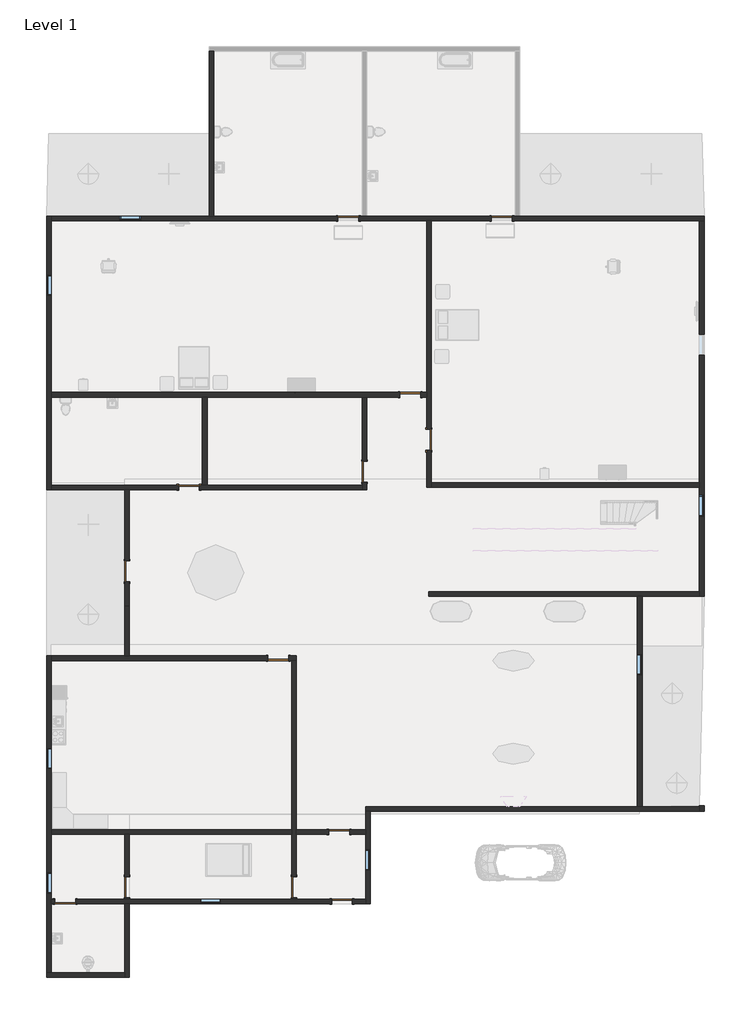
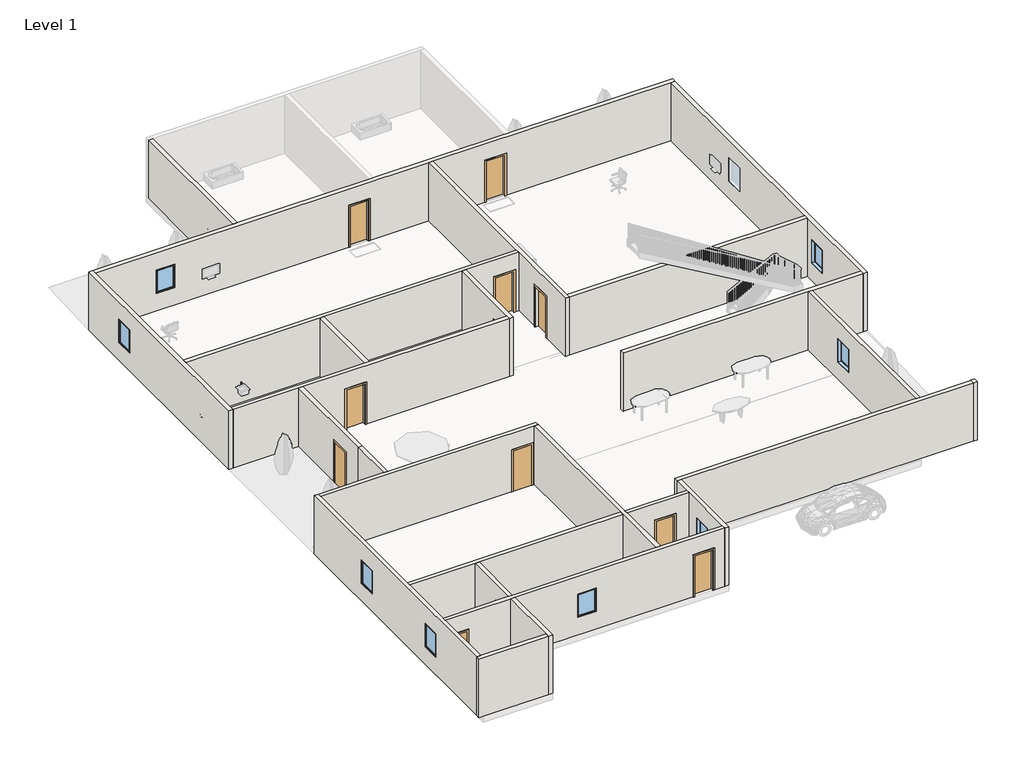
# One storey, part 1 of 4: 26 walls, 13 doors, 8 windows.
"""IFC4 building model written with IfcOpenShell, lengths in millimetres."""

from ifc_helpers import new_model, si_unit, frame, origin, origin_with_axes, place, context, project, spatial, polyline, outline, extrude, faceted_brep, transform, mapped, element, save
from components import door_54dd4da4, door_719f80de, window_e2841890

model = new_model("IFC4")

# Units and contexts
model_context = context("Model", 3, world=origin())
ifc_project = project(units=[si_unit("LENGTHUNIT", "METRE", prefix="MILLI")], contexts=[model_context])

# Site, building, storey
site = spatial("IfcSite", under=ifc_project)
building = spatial("IfcBuilding", under=site)
storey = spatial("IfcBuildingStorey", under=building, Name="Level 1", Elevation=0.0)

# Doors
placement = place(None, origin())
door_shape = door_54dd4da4(model_context)
element("IfcDoor", 1, ObjectType="Single-Flush : 36\" x 84\"", at=placement, inside=storey, context=model_context, shape_type="MappedRepresentation", body=[
    mapped(door_shape, transform((512.5171827, 13399.1665396, 0.0), x_axis=(1.0, 0.0, 0.0), y_axis=(0.0, 1.0, 0.0), z_axis=(0.0, 0.0, 1.0))),
])
element("IfcDoor", 2, ObjectType="Single-Flush : 36\" x 84\"", at=placement, inside=storey, context=model_context, shape_type="MappedRepresentation", body=[
    mapped(door_shape, transform((7243.5171827, 13399.1665396, 0.0), x_axis=(1.0, 0.0, 0.0), y_axis=(0.0, 1.0, 0.0), z_axis=(0.0, 0.0, 1.0))),
])
element("IfcDoor", 3, ObjectType="Single-Flush : 36\" x 84\"", at=placement, inside=storey, context=model_context, shape_type="MappedRepresentation", body=[
    mapped(door_shape, transform((3230.3171827, 5677.5665396, 0.0), x_axis=(1.0, 0.0, 0.0), y_axis=(0.0, 1.0, 0.0), z_axis=(0.0, 0.0, 1.0))),
])
element("IfcDoor", 4, ObjectType="Single-Flush : 36\" x 84\"", at=placement, inside=storey, context=model_context, shape_type="MappedRepresentation", body=[
    mapped(door_shape, transform((4043.1171827, 3696.3665396, 0.0), x_axis=(0.0, -1.0, 0.0), y_axis=(1.0, 0.0, 0.0), z_axis=(0.0, 0.0, 1.0))),
])
element("IfcDoor", 5, ObjectType="Single-Flush : 36\" x 84\"", at=placement, inside=storey, context=model_context, shape_type="MappedRepresentation", body=[
    mapped(door_shape, transform((-6472.4828173, 1613.5665396, 0.0), x_axis=(1.0, 0.0, 0.0), y_axis=(0.0, 1.0, 0.0), z_axis=(0.0, 0.0, 1.0))),
])
element("IfcDoor", 6, ObjectType="Single-Flush : 36\" x 84\"", at=placement, inside=storey, context=model_context, shape_type="MappedRepresentation", body=[
    mapped(door_shape, transform((-11908.0828173, -16547.4334604, 0.0), x_axis=(-1.0, 0.0, 0.0), y_axis=(0.0, -1.0, 0.0), z_axis=(0.0, 0.0, 1.0))),
])
element("IfcDoor", 7, ObjectType="Single-Flush : 36\" x 84\"", at=placement, inside=storey, context=model_context, shape_type="MappedRepresentation", body=[
    mapped(door_shape, transform((233.1171827, -16547.4334604, 0.0), x_axis=(1.0, 0.0, 0.0), y_axis=(0.0, 1.0, 0.0), z_axis=(0.0, 0.0, 1.0))),
])
element("IfcDoor", 8, ObjectType="Single-Flush : 36\" x 84\"", at=placement, inside=storey, context=model_context, shape_type="MappedRepresentation", body=[
    mapped(door_shape, transform((-9190.2828173, -2069.4334604, 0.0), x_axis=(0.0, 1.0, 0.0), y_axis=(-1.0, 0.0, 0.0), z_axis=(0.0, 0.0, 1.0))),
])
door_2_shape = door_719f80de(model_context)
element("IfcDoor", 9, ObjectType="Single-Flush : 36\" x 84\"", at=placement, inside=storey, context=model_context, shape_type="MappedRepresentation", body=[
    mapped(door_2_shape, transform((1223.7171827, 2299.3665396, 0.0), x_axis=(0.0, -1.0, 0.0), y_axis=(1.0, 0.0, 0.0), z_axis=(0.0, 0.0, 1.0))),
])
element("IfcDoor", 10, ObjectType="Single-Flush : 36\" x 84\"", at=placement, inside=storey, context=model_context, shape_type="MappedRepresentation", body=[
    mapped(door_2_shape, transform((-2560.8828173, -5879.4334604, 0.0), x_axis=(1.0, 0.0, 0.0), y_axis=(0.0, 1.0, 0.0), z_axis=(0.0, 0.0, 1.0))),
])
element("IfcDoor", 11, ObjectType="Single-Flush : 36\" x 84\"", at=placement, inside=storey, context=model_context, shape_type="MappedRepresentation", body=[
    mapped(door_2_shape, transform((-9190.2828173, -15912.4334604, 0.0), x_axis=(0.0, -1.0, 0.0), y_axis=(1.0, 0.0, 0.0), z_axis=(0.0, 0.0, 1.0))),
])
element("IfcDoor", 12, ObjectType="Single-Flush : 36\" x 84\"", at=placement, inside=storey, context=model_context, shape_type="MappedRepresentation", body=[
    mapped(door_2_shape, transform((-1875.0828173, -15912.4334604, 0.0), x_axis=(0.0, -1.0, 0.0), y_axis=(1.0, 0.0, 0.0), z_axis=(0.0, 0.0, 1.0))),
])
element("IfcDoor", 13, ObjectType="Single-Flush : 36\" x 84\"", at=placement, inside=storey, context=model_context, shape_type="MappedRepresentation", body=[
    mapped(door_2_shape, transform((106.1171827, -13499.4334604, 0.0), x_axis=(-1.0, 0.0, 0.0), y_axis=(0.0, -1.0, 0.0), z_axis=(0.0, 0.0, 1.0))),
])

# Walls
element("IfcWall", 14, ObjectType="Generic - 8\"", at=placement, inside=storey, context=model_context, shape_type="SweptSolid", body=[
    extrude(outline(polyline([(-5583.4828173, 13500.7665396), (-5583.4828173, 20739.7665396), (-5380.2828173, 20739.7665396), (-5380.2828173, 13500.7665396), (-5583.4828173, 13500.7665396)])), origin_with_axes(), (0.0, 0.0, 1.0), 3048.0),
])
element("IfcWall", 15, ObjectType="Generic - 8\"", at=placement, inside=storey, context=model_context, shape_type="Brep", body=[
    faceted_brep([(7700.7171827, 13297.5665396, 2133.6), (7700.7171827, 13297.5665396, 0.0), (15904.9171827, 13297.5665396, 0.0), (16108.1171827, 13297.5665396, 0.0), (16108.1171827, 13297.5665396, 3048.0), (15904.9171827, 13297.5665396, 3048.0), (4144.7171827, 13297.5665396, 3048.0), (3941.5171827, 13297.5665396, 3048.0), (-12517.6828173, 13297.5665396, 3048.0), (-12517.6828173, 13297.5665396, 0.0), (55.3171827, 13297.5665396, 0.0), (55.3171827, 13297.5665396, 2133.6), (969.7171827, 13297.5665396, 2133.6), (969.7171827, 13297.5665396, 0.0), (3941.5171827, 13297.5665396, 0.0), (4144.7171827, 13297.5665396, 0.0), (6786.3171827, 13297.5665396, 0.0), (6786.3171827, 13297.5665396, 2133.6), (-9507.7828173, 13297.5665396, 2133.6), (-8593.3828173, 13297.5665396, 2133.6), (-8593.3828173, 13297.5665396, 914.4), (-9507.7828173, 13297.5665396, 914.4), (16108.1171827, 13500.7665396, 0.0), (8030.9171827, 13500.7665396, 0.0), (7827.7171827, 13500.7665396, 0.0), (7700.7171827, 13500.7665396, 0.0), (7700.7171827, 13500.7665396, 2133.6), (6786.3171827, 13500.7665396, 2133.6), (6786.3171827, 13500.7665396, 0.0), (1325.3171827, 13500.7665396, 0.0), (1122.1171827, 13500.7665396, 0.0), (969.7171827, 13500.7665396, 0.0), (969.7171827, 13500.7665396, 2133.6), (55.3171827, 13500.7665396, 2133.6), (55.3171827, 13500.7665396, 0.0), (-5380.2828173, 13500.7665396, 0.0), (-5583.4828173, 13500.7665396, 0.0), (-12517.6828173, 13500.7665396, 0.0), (-12517.6828173, 13500.7665396, 3048.0), (-5583.4828173, 13500.7665396, 3048.0), (-5380.2828173, 13500.7665396, 3048.0), (1122.1171827, 13500.7665396, 3048.0), (1325.3171827, 13500.7665396, 3048.0), (7827.7171827, 13500.7665396, 3048.0), (8030.9171827, 13500.7665396, 3048.0), (16108.1171827, 13500.7665396, 3048.0), (-9507.7828173, 13500.7665396, 2133.6), (-9507.7828173, 13500.7665396, 914.4), (-8593.3828173, 13500.7665396, 914.4), (-8593.3828173, 13500.7665396, 2133.6)], [[[0, 1, 2, 3, 4, 5, 6, 7, 8, 9, 10, 11, 12, 13, 14, 15, 16, 17], [18, 19, 20, 21]], [[22, 23, 24, 25, 26, 27, 28, 29, 30, 31, 32, 33, 34, 35, 36, 37, 38, 39, 40, 41, 42, 43, 44, 45], [46, 47, 48, 49]], [[10, 9, 37, 36, 35, 34]], [[3, 2, 1, 25, 24, 23, 22]], [[16, 15, 14, 13, 31, 30, 29, 28]], [[8, 7, 6, 5, 4, 45, 44, 43, 42, 41, 40, 39, 38]], [[4, 3, 22, 45]], [[9, 8, 38, 37]], [[32, 31, 13, 12]], [[33, 32, 12, 11]], [[34, 33, 11, 10]], [[26, 25, 1, 0]], [[27, 26, 0, 17]], [[28, 27, 17, 16]], [[47, 46, 18, 21]], [[48, 47, 21, 20]], [[49, 48, 20, 19]], [[46, 49, 19, 18]]]),
])
element("IfcWall", 16, ObjectType="Generic - 8\"", at=placement, inside=storey, context=model_context, shape_type="Brep", body=[
    faceted_brep([(15904.9171827, 13297.5665396, 0.0), (15904.9171827, 1816.7665396, 0.0), (15904.9171827, 1613.5665396, 0.0), (15904.9171827, -2958.4334604, 0.0), (15904.9171827, -3161.6334604, 0.0), (15904.9171827, -3161.6334604, 3048.0), (15904.9171827, -2958.4334604, 3048.0), (15904.9171827, 1613.5665396, 3048.0), (15904.9171827, 1816.7665396, 3048.0), (15904.9171827, 13297.5665396, 3048.0), (15904.9171827, 343.5665396, 2133.6), (15904.9171827, 343.5665396, 914.4), (15904.9171827, 1257.9665396, 914.4), (15904.9171827, 1257.9665396, 2133.6), (15904.9171827, 7404.7665396, 2133.6), (15904.9171827, 7404.7665396, 914.4), (15904.9171827, 8319.1665396, 914.4), (15904.9171827, 8319.1665396, 2133.6), (16108.1171827, 13297.5665396, 0.0), (16108.1171827, 13297.5665396, 3048.0), (16108.1171827, -3161.6334604, 3048.0), (16108.1171827, -3161.6334604, 0.0), (16108.1171827, 343.5665396, 2133.6), (16108.1171827, 1257.9665396, 2133.6), (16108.1171827, 1257.9665396, 914.4), (16108.1171827, 343.5665396, 914.4), (16108.1171827, 7404.7665396, 2133.6), (16108.1171827, 8319.1665396, 2133.6), (16108.1171827, 8319.1665396, 914.4), (16108.1171827, 7404.7665396, 914.4)], [[[0, 1, 2, 3, 4, 5, 6, 7, 8, 9], [10, 11, 12, 13], [14, 15, 16, 17]], [[18, 19, 20, 21], [22, 23, 24, 25], [26, 27, 28, 29]], [[4, 3, 2, 1, 0, 18, 21]], [[9, 8, 7, 6, 5, 20, 19]], [[0, 9, 19, 18]], [[11, 10, 22, 25]], [[12, 11, 25, 24]], [[13, 12, 24, 23]], [[10, 13, 23, 22]], [[15, 14, 26, 29]], [[16, 15, 29, 28]], [[17, 16, 28, 27]], [[14, 17, 27, 26]], [[5, 4, 21, 20]]]),
])
element("IfcWall", 17, ObjectType="Generic - 8\"", at=placement, inside=storey, context=model_context, shape_type="Brep", body=[
    faceted_brep([(15904.9171827, -12381.8334604, 0.0), (13390.3171827, -12381.8334604, 0.0), (13187.1171827, -12381.8334604, 0.0), (1274.5171827, -12381.8334604, 0.0), (1274.5171827, -12381.8334604, 3048.0), (13187.1171827, -12381.8334604, 3048.0), (13390.3171827, -12381.8334604, 3048.0), (15904.9171827, -12381.8334604, 3048.0), (15904.9171827, -12585.0334604, 0.0), (15904.9171827, -12585.0334604, 3048.0), (1477.7171827, -12585.0334604, 3048.0), (1274.5171827, -12585.0334604, 3048.0), (1274.5171827, -12585.0334604, 0.0), (1477.7171827, -12585.0334604, 0.0)], [[[0, 1, 2, 3, 4, 5, 6, 7]], [[8, 9, 10, 11, 12, 13]], [[3, 2, 1, 0, 8, 13, 12]], [[7, 6, 5, 4, 11, 10, 9]], [[0, 7, 9, 8]], [[4, 3, 12, 11]]]),
])
element("IfcWall", 18, ObjectType="Generic - 8\"", at=placement, inside=storey, context=model_context, shape_type="Brep", body=[
    faceted_brep([(1274.5171827, -12585.0334604, 0.0), (1274.5171827, -13397.8334604, 0.0), (1274.5171827, -13601.0334604, 0.0), (1274.5171827, -16445.8334604, 0.0), (1274.5171827, -16649.0334604, 0.0), (1274.5171827, -16649.0334604, 3048.0), (1274.5171827, -16445.8334604, 3048.0), (1274.5171827, -13601.0334604, 3048.0), (1274.5171827, -13397.8334604, 3048.0), (1274.5171827, -12585.0334604, 3048.0), (1274.5171827, -15175.8334604, 2133.6), (1274.5171827, -15175.8334604, 914.4), (1274.5171827, -14261.4334604, 914.4), (1274.5171827, -14261.4334604, 2133.6), (1477.7171827, -12585.0334604, 0.0), (1477.7171827, -12585.0334604, 3048.0), (1477.7171827, -16649.0334604, 3048.0), (1477.7171827, -16649.0334604, 0.0), (1477.7171827, -15175.8334604, 2133.6), (1477.7171827, -14261.4334604, 2133.6), (1477.7171827, -14261.4334604, 914.4), (1477.7171827, -15175.8334604, 914.4)], [[[0, 1, 2, 3, 4, 5, 6, 7, 8, 9], [10, 11, 12, 13]], [[14, 15, 16, 17], [18, 19, 20, 21]], [[4, 3, 2, 1, 0, 14, 17]], [[9, 8, 7, 6, 5, 16, 15]], [[0, 9, 15, 14]], [[5, 4, 17, 16]], [[11, 10, 18, 21]], [[12, 11, 21, 20]], [[13, 12, 20, 19]], [[10, 13, 19, 18]]]),
])
element("IfcWall", 19, ObjectType="Generic - 8\"", at=placement, inside=storey, context=model_context, shape_type="Brep", body=[
    faceted_brep([(1274.5171827, -16445.8334604, 0.0), (690.3171827, -16445.8334604, 0.0), (690.3171827, -16445.8334604, 2133.6), (-224.0828173, -16445.8334604, 2133.6), (-224.0828173, -16445.8334604, 0.0), (-1773.4828173, -16445.8334604, 0.0), (-1976.6828173, -16445.8334604, 0.0), (-9088.6828173, -16445.8334604, 0.0), (-9291.8828173, -16445.8334604, 0.0), (-11450.8828173, -16445.8334604, 0.0), (-11450.8828173, -16445.8334604, 2133.6), (-12365.2828173, -16445.8334604, 2133.6), (-12365.2828173, -16445.8334604, 0.0), (-12517.6828173, -16445.8334604, 0.0), (-12517.6828173, -16445.8334604, 3048.0), (-9291.8828173, -16445.8334604, 3048.0), (-9088.6828173, -16445.8334604, 3048.0), (-1976.6828173, -16445.8334604, 3048.0), (-1773.4828173, -16445.8334604, 3048.0), (1274.5171827, -16445.8334604, 3048.0), (-5989.8828173, -16445.8334604, 2133.6), (-5989.8828173, -16445.8334604, 914.4), (-5075.4828173, -16445.8334604, 914.4), (-5075.4828173, -16445.8334604, 2133.6), (690.3171827, -16649.0334604, 2133.6), (690.3171827, -16649.0334604, 0.0), (1274.5171827, -16649.0334604, 0.0), (1274.5171827, -16649.0334604, 3048.0), (-9088.6828173, -16649.0334604, 3048.0), (-9291.8828173, -16649.0334604, 3048.0), (-12517.6828173, -16649.0334604, 3048.0), (-12517.6828173, -16649.0334604, 0.0), (-12365.2828173, -16649.0334604, 0.0), (-12365.2828173, -16649.0334604, 2133.6), (-11450.8828173, -16649.0334604, 2133.6), (-11450.8828173, -16649.0334604, 0.0), (-9291.8828173, -16649.0334604, 0.0), (-9088.6828173, -16649.0334604, 0.0), (-224.0828173, -16649.0334604, 0.0), (-224.0828173, -16649.0334604, 2133.6), (-5989.8828173, -16649.0334604, 2133.6), (-5075.4828173, -16649.0334604, 2133.6), (-5075.4828173, -16649.0334604, 914.4), (-5989.8828173, -16649.0334604, 914.4)], [[[0, 1, 2, 3, 4, 5, 6, 7, 8, 9, 10, 11, 12, 13, 14, 15, 16, 17, 18, 19], [20, 21, 22, 23]], [[24, 25, 26, 27, 28, 29, 30, 31, 32, 33, 34, 35, 36, 37, 38, 39], [40, 41, 42, 43]], [[13, 12, 32, 31]], [[26, 25, 1, 0]], [[38, 37, 36, 35, 9, 8, 7, 6, 5, 4]], [[19, 18, 17, 16, 15, 14, 30, 29, 28, 27]], [[0, 19, 27, 26]], [[14, 13, 31, 30]], [[21, 20, 40, 43]], [[22, 21, 43, 42]], [[23, 22, 42, 41]], [[20, 23, 41, 40]], [[33, 32, 12, 11]], [[34, 33, 11, 10]], [[35, 34, 10, 9]], [[2, 1, 25, 24]], [[3, 2, 24, 39]], [[4, 3, 39, 38]]]),
])
element("IfcWall", 20, ObjectType="Generic - 8\"", at=placement, inside=storey, context=model_context, shape_type="Brep", body=[
    faceted_brep([(-9291.8828173, -16649.0334604, 0.0), (-9291.8828173, -19671.6334604, 0.0), (-9291.8828173, -19874.8334604, 0.0), (-9291.8828173, -19874.8334604, 3048.0), (-9291.8828173, -19671.6334604, 3048.0), (-9291.8828173, -16649.0334604, 3048.0), (-9088.6828173, -16649.0334604, 0.0), (-9088.6828173, -16649.0334604, 3048.0), (-9088.6828173, -19874.8334604, 3048.0), (-9088.6828173, -19874.8334604, 0.0)], [[[0, 1, 2, 3, 4, 5]], [[6, 7, 8, 9]], [[2, 1, 0, 6, 9]], [[5, 4, 3, 8, 7]], [[0, 5, 7, 6]], [[3, 2, 9, 8]]]),
])
element("IfcWall", 21, ObjectType="Generic - 8\"", at=placement, inside=storey, context=model_context, shape_type="Brep", body=[
    faceted_brep([(-9291.8828173, -19671.6334604, 0.0), (-12517.6828173, -19671.6334604, 0.0), (-12720.8828173, -19671.6334604, 0.0), (-12720.8828173, -19671.6334604, 3048.0), (-12517.6828173, -19671.6334604, 3048.0), (-9291.8828173, -19671.6334604, 3048.0), (-9291.8828173, -19874.8334604, 0.0), (-9291.8828173, -19874.8334604, 3048.0), (-12720.8828173, -19874.8334604, 3048.0), (-12720.8828173, -19874.8334604, 0.0)], [[[0, 1, 2, 3, 4, 5]], [[6, 7, 8, 9]], [[2, 1, 0, 6, 9]], [[5, 4, 3, 8, 7]], [[0, 5, 7, 6]], [[3, 2, 9, 8]]]),
])
element("IfcWall", 22, ObjectType="Generic - 8\"", at=placement, inside=storey, context=model_context, shape_type="Brep", body=[
    faceted_brep([(-12517.6828173, -19671.6334604, 0.0), (-12517.6828173, -16649.0334604, 0.0), (-12517.6828173, -16445.8334604, 0.0), (-12517.6828173, -13601.0334604, 0.0), (-12517.6828173, -13397.8334604, 0.0), (-12517.6828173, -5981.0334604, 0.0), (-12517.6828173, -5777.8334604, 0.0), (-12517.6828173, -5777.8334604, 3048.0), (-12517.6828173, -5981.0334604, 3048.0), (-12517.6828173, -13397.8334604, 3048.0), (-12517.6828173, -13601.0334604, 3048.0), (-12517.6828173, -16445.8334604, 3048.0), (-12517.6828173, -16649.0334604, 3048.0), (-12517.6828173, -19671.6334604, 3048.0), (-12517.6828173, -9816.4334604, 2133.6), (-12517.6828173, -9816.4334604, 914.4), (-12517.6828173, -10730.8334604, 914.4), (-12517.6828173, -10730.8334604, 2133.6), (-12517.6828173, -15277.4334604, 2133.6), (-12517.6828173, -15277.4334604, 914.4), (-12517.6828173, -16191.8334604, 914.4), (-12517.6828173, -16191.8334604, 2133.6), (-12720.8828173, -19671.6334604, 0.0), (-12720.8828173, -19671.6334604, 3048.0), (-12720.8828173, -5777.8334604, 3048.0), (-12720.8828173, -5777.8334604, 0.0), (-12720.8828173, -9816.4334604, 2133.6), (-12720.8828173, -10730.8334604, 2133.6), (-12720.8828173, -10730.8334604, 914.4), (-12720.8828173, -9816.4334604, 914.4), (-12720.8828173, -15277.4334604, 2133.6), (-12720.8828173, -16191.8334604, 2133.6), (-12720.8828173, -16191.8334604, 914.4), (-12720.8828173, -15277.4334604, 914.4)], [[[0, 1, 2, 3, 4, 5, 6, 7, 8, 9, 10, 11, 12, 13], [14, 15, 16, 17], [18, 19, 20, 21]], [[22, 23, 24, 25], [26, 27, 28, 29], [30, 31, 32, 33]], [[6, 5, 4, 3, 2, 1, 0, 22, 25]], [[13, 12, 11, 10, 9, 8, 7, 24, 23]], [[0, 13, 23, 22]], [[15, 14, 26, 29]], [[16, 15, 29, 28]], [[17, 16, 28, 27]], [[14, 17, 27, 26]], [[19, 18, 30, 33]], [[20, 19, 33, 32]], [[21, 20, 32, 31]], [[18, 21, 31, 30]], [[7, 6, 25, 24]]]),
])
element("IfcWall", 23, ObjectType="Generic - 8\"", at=placement, inside=storey, context=model_context, shape_type="Brep", body=[
    faceted_brep([(3687.5171827, 5575.9665396, 2133.6), (3687.5171827, 5575.9665396, 0.0), (3941.5171827, 5575.9665396, 0.0), (3941.5171827, 5575.9665396, 3048.0), (1325.3171827, 5575.9665396, 3048.0), (1122.1171827, 5575.9665396, 3048.0), (-5685.0828173, 5575.9665396, 3048.0), (-5888.2828173, 5575.9665396, 3048.0), (-12517.6828173, 5575.9665396, 3048.0), (-12517.6828173, 5575.9665396, 0.0), (-5888.2828173, 5575.9665396, 0.0), (-5685.0828173, 5575.9665396, 0.0), (1122.1171827, 5575.9665396, 0.0), (1325.3171827, 5575.9665396, 0.0), (2773.1171827, 5575.9665396, 0.0), (2773.1171827, 5575.9665396, 2133.6), (3941.5171827, 5779.1665396, 0.0), (3687.5171827, 5779.1665396, 0.0), (3687.5171827, 5779.1665396, 2133.6), (2773.1171827, 5779.1665396, 2133.6), (2773.1171827, 5779.1665396, 0.0), (-12517.6828173, 5779.1665396, 0.0), (-12517.6828173, 5779.1665396, 3048.0), (3941.5171827, 5779.1665396, 3048.0)], [[[0, 1, 2, 3, 4, 5, 6, 7, 8, 9, 10, 11, 12, 13, 14, 15]], [[16, 17, 18, 19, 20, 21, 22, 23]], [[2, 1, 17, 16]], [[14, 13, 12, 11, 10, 9, 21, 20]], [[8, 7, 6, 5, 4, 3, 23, 22]], [[9, 8, 22, 21]], [[3, 2, 16, 23]], [[18, 17, 1, 0]], [[19, 18, 0, 15]], [[20, 19, 15, 14]]]),
])
element("IfcWall", 24, ObjectType="Generic - 8\"", at=placement, inside=storey, context=model_context, shape_type="Brep", body=[
    faceted_brep([(4144.7171827, 1613.5665396, 0.0), (4144.7171827, 1816.7665396, 0.0), (4144.7171827, 3239.1665396, 0.0), (4144.7171827, 3239.1665396, 2133.6), (4144.7171827, 4153.5665396, 2133.6), (4144.7171827, 4153.5665396, 0.0), (4144.7171827, 13297.5665396, 0.0), (4144.7171827, 13297.5665396, 3048.0), (4144.7171827, 1816.7665396, 3048.0), (4144.7171827, 1613.5665396, 3048.0), (3941.5171827, 3239.1665396, 2133.6), (3941.5171827, 3239.1665396, 0.0), (3941.5171827, 1613.5665396, 0.0), (3941.5171827, 1613.5665396, 3048.0), (3941.5171827, 5575.9665396, 3048.0), (3941.5171827, 5779.1665396, 3048.0), (3941.5171827, 13297.5665396, 3048.0), (3941.5171827, 13297.5665396, 0.0), (3941.5171827, 5779.1665396, 0.0), (3941.5171827, 5575.9665396, 0.0), (3941.5171827, 4153.5665396, 0.0), (3941.5171827, 4153.5665396, 2133.6)], [[[0, 1, 2, 3, 4, 5, 6, 7, 8, 9]], [[10, 11, 12, 13, 14, 15, 16, 17, 18, 19, 20, 21]], [[12, 11, 2, 1, 0]], [[20, 19, 18, 17, 6, 5]], [[9, 8, 7, 16, 15, 14, 13]], [[7, 6, 17, 16]], [[0, 9, 13, 12]], [[3, 2, 11, 10]], [[4, 3, 10, 21]], [[5, 4, 21, 20]]]),
])
element("IfcWall", 25, ObjectType="Generic - 8\"", at=placement, inside=storey, context=model_context, shape_type="Brep", body=[
    faceted_brep([(1122.1171827, 1842.1665396, 2133.6), (1122.1171827, 1842.1665396, 0.0), (1122.1171827, 1715.1665396, 0.0), (1122.1171827, 1511.9665396, 0.0), (1122.1171827, 1511.9665396, 3048.0), (1122.1171827, 1715.1665396, 3048.0), (1122.1171827, 5575.9665396, 3048.0), (1122.1171827, 5575.9665396, 0.0), (1122.1171827, 2756.5665396, 0.0), (1122.1171827, 2756.5665396, 2133.6), (1325.3171827, 1511.9665396, 0.0), (1325.3171827, 1842.1665396, 0.0), (1325.3171827, 1842.1665396, 2133.6), (1325.3171827, 2756.5665396, 2133.6), (1325.3171827, 2756.5665396, 0.0), (1325.3171827, 5575.9665396, 0.0), (1325.3171827, 5575.9665396, 3048.0), (1325.3171827, 1511.9665396, 3048.0)], [[[0, 1, 2, 3, 4, 5, 6, 7, 8, 9]], [[10, 11, 12, 13, 14, 15, 16, 17]], [[8, 7, 15, 14]], [[3, 2, 1, 11, 10]], [[6, 5, 4, 17, 16]], [[7, 6, 16, 15]], [[4, 3, 10, 17]], [[12, 11, 1, 0]], [[13, 12, 0, 9]], [[14, 13, 9, 8]]]),
])
element("IfcWall", 26, ObjectType="Generic - 8\"", at=placement, inside=storey, context=model_context, shape_type="Brep", body=[
    faceted_brep([(1122.1171827, 1715.1665396, 0.0), (-5685.0828173, 1715.1665396, 0.0), (-5888.2828173, 1715.1665396, 0.0), (-6015.2828173, 1715.1665396, 0.0), (-6015.2828173, 1715.1665396, 2133.6), (-6929.6828173, 1715.1665396, 2133.6), (-6929.6828173, 1715.1665396, 0.0), (-12517.6828173, 1715.1665396, 0.0), (-12517.6828173, 1715.1665396, 3048.0), (-5888.2828173, 1715.1665396, 3048.0), (-5685.0828173, 1715.1665396, 3048.0), (1122.1171827, 1715.1665396, 3048.0), (-6015.2828173, 1511.9665396, 2133.6), (-6015.2828173, 1511.9665396, 0.0), (1122.1171827, 1511.9665396, 0.0), (1122.1171827, 1511.9665396, 3048.0), (-9088.6828173, 1511.9665396, 3048.0), (-9291.8828173, 1511.9665396, 3048.0), (-12517.6828173, 1511.9665396, 3048.0), (-12517.6828173, 1511.9665396, 0.0), (-9291.8828173, 1511.9665396, 0.0), (-9088.6828173, 1511.9665396, 0.0), (-6929.6828173, 1511.9665396, 0.0), (-6929.6828173, 1511.9665396, 2133.6)], [[[0, 1, 2, 3, 4, 5, 6, 7, 8, 9, 10, 11]], [[12, 13, 14, 15, 16, 17, 18, 19, 20, 21, 22, 23]], [[14, 13, 3, 2, 1, 0]], [[22, 21, 20, 19, 7, 6]], [[11, 10, 9, 8, 18, 17, 16, 15]], [[0, 11, 15, 14]], [[4, 3, 13, 12]], [[5, 4, 12, 23]], [[6, 5, 23, 22]], [[8, 7, 19, 18]]]),
])
element("IfcWall", 27, ObjectType="Generic - 8\"", at=placement, inside=storey, context=model_context, shape_type="SweptSolid", body=[
    extrude(outline(polyline([(1511.9665396, 0.0), (-1612.2334604, 0.0), (-1612.2334604, 2133.6), (-2526.6334604, 2133.6), (-2526.6334604, 0.0), (-3593.4334604, 0.0), (-3593.4334604, 3048.0), (1511.9665396, 3048.0), (1511.9665396, 0.0)])), frame((-9291.8828173, 0.0, 0.0), z_axis=(1.0, 0.0, 0.0), x_axis=(0.0, 1.0, 0.0)), (0.0, 0.0, 1.0), 203.2),
])
element("IfcWall", 28, ObjectType="Generic - 8\"", at=placement, inside=storey, context=model_context, shape_type="Brep", body=[
    faceted_brep([(-1773.4828173, -5777.8334604, 0.0), (-2103.6828173, -5777.8334604, 0.0), (-2103.6828173, -5777.8334604, 2133.6), (-3018.0828173, -5777.8334604, 2133.6), (-3018.0828173, -5777.8334604, 0.0), (-9088.6828173, -5777.8334604, 0.0), (-9291.8828173, -5777.8334604, 0.0), (-12517.6828173, -5777.8334604, 0.0), (-12517.6828173, -5777.8334604, 3048.0), (-9291.8828173, -5777.8334604, 3048.0), (-9088.6828173, -5777.8334604, 3048.0), (-1773.4828173, -5777.8334604, 3048.0), (-2103.6828173, -5981.0334604, 2133.6), (-2103.6828173, -5981.0334604, 0.0), (-1976.6828173, -5981.0334604, 0.0), (-1773.4828173, -5981.0334604, 0.0), (-1773.4828173, -5981.0334604, 3048.0), (-1976.6828173, -5981.0334604, 3048.0), (-12517.6828173, -5981.0334604, 3048.0), (-12517.6828173, -5981.0334604, 0.0), (-3018.0828173, -5981.0334604, 0.0), (-3018.0828173, -5981.0334604, 2133.6)], [[[0, 1, 2, 3, 4, 5, 6, 7, 8, 9, 10, 11]], [[12, 13, 14, 15, 16, 17, 18, 19, 20, 21]], [[20, 19, 7, 6, 5, 4]], [[15, 14, 13, 1, 0]], [[11, 10, 9, 8, 18, 17, 16]], [[0, 11, 16, 15]], [[2, 1, 13, 12]], [[3, 2, 12, 21]], [[4, 3, 21, 20]], [[8, 7, 19, 18]]]),
])
element("IfcWall", 29, ObjectType="Generic - 8\"", at=placement, inside=storey, context=model_context, shape_type="Brep", body=[
    faceted_brep([(-1976.6828173, -16369.6334604, 2133.6), (-1976.6828173, -16369.6334604, 0.0), (-1976.6828173, -16445.8334604, 0.0), (-1976.6828173, -16445.8334604, 3048.0), (-1976.6828173, -13601.0334604, 3048.0), (-1976.6828173, -13397.8334604, 3048.0), (-1976.6828173, -5981.0334604, 3048.0), (-1976.6828173, -5981.0334604, 0.0), (-1976.6828173, -13397.8334604, 0.0), (-1976.6828173, -13601.0334604, 0.0), (-1976.6828173, -15455.2334604, 0.0), (-1976.6828173, -15455.2334604, 2133.6), (-1773.4828173, -16445.8334604, 0.0), (-1773.4828173, -16369.6334604, 0.0), (-1773.4828173, -16369.6334604, 2133.6), (-1773.4828173, -15455.2334604, 2133.6), (-1773.4828173, -15455.2334604, 0.0), (-1773.4828173, -13601.0334604, 0.0), (-1773.4828173, -13397.8334604, 0.0), (-1773.4828173, -5981.0334604, 0.0), (-1773.4828173, -5981.0334604, 3048.0), (-1773.4828173, -13397.8334604, 3048.0), (-1773.4828173, -13601.0334604, 3048.0), (-1773.4828173, -16445.8334604, 3048.0)], [[[0, 1, 2, 3, 4, 5, 6, 7, 8, 9, 10, 11]], [[12, 13, 14, 15, 16, 17, 18, 19, 20, 21, 22, 23]], [[2, 1, 13, 12]], [[10, 9, 8, 7, 19, 18, 17, 16]], [[6, 5, 4, 3, 23, 22, 21, 20]], [[7, 6, 20, 19]], [[3, 2, 12, 23]], [[14, 13, 1, 0]], [[15, 14, 0, 11]], [[16, 15, 11, 10]]]),
])
element("IfcWall", 30, ObjectType="Generic - 8\"", at=placement, inside=storey, context=model_context, shape_type="Brep", body=[
    faceted_brep([(-1976.6828173, -13397.8334604, 0.0), (-12517.6828173, -13397.8334604, 0.0), (-12517.6828173, -13397.8334604, 3048.0), (-1976.6828173, -13397.8334604, 3048.0), (-1976.6828173, -13601.0334604, 0.0), (-1976.6828173, -13601.0334604, 3048.0), (-9088.6828173, -13601.0334604, 3048.0), (-9291.8828173, -13601.0334604, 3048.0), (-12517.6828173, -13601.0334604, 3048.0), (-12517.6828173, -13601.0334604, 0.0), (-9291.8828173, -13601.0334604, 0.0), (-9088.6828173, -13601.0334604, 0.0)], [[[0, 1, 2, 3]], [[4, 5, 6, 7, 8, 9, 10, 11]], [[1, 0, 4, 11, 10, 9]], [[3, 2, 8, 7, 6, 5]], [[2, 1, 9, 8]], [[0, 3, 5, 4]]]),
])
element("IfcWall", 31, ObjectType="Generic - 8\"", at=placement, inside=storey, context=model_context, shape_type="SweptSolid", body=[
    extrude(outline(polyline([(-16369.6334604, 2133.6), (-16369.6334604, 0.0), (-16445.8334604, 0.0), (-16445.8334604, 3048.0), (-13601.0334604, 3048.0), (-13601.0334604, 0.0), (-15455.2334604, 0.0), (-15455.2334604, 2133.6), (-16369.6334604, 2133.6)])), frame((-9291.8828173, 0.0, 0.0), z_axis=(1.0, 0.0, 0.0), x_axis=(0.0, 1.0, 0.0)), (0.0, 0.0, 1.0), 203.2),
])
element("IfcWall", 32, ObjectType="Generic - 8\"", at=placement, inside=storey, context=model_context, shape_type="SweptSolid", body=[
    extrude(outline(polyline([(4144.7171827, 1816.7665396), (15904.9171827, 1816.7665396), (15904.9171827, 1613.5665396), (4144.7171827, 1613.5665396), (4144.7171827, 1816.7665396)])), origin_with_axes(), (0.0, 0.0, 1.0), 3048.0),
])
element("IfcWall", 33, ObjectType="Generic - 8\"", at=placement, inside=storey, context=model_context, shape_type="Brep", body=[
    faceted_brep([(15904.9171827, -2958.4334604, 0.0), (4043.1171827, -2958.4334604, 0.0), (4043.1171827, -2958.4334604, 3048.0), (15904.9171827, -2958.4334604, 3048.0), (15904.9171827, -3161.6334604, 0.0), (15904.9171827, -3161.6334604, 3048.0), (13390.3171827, -3161.6334604, 3048.0), (13187.1171827, -3161.6334604, 3048.0), (4043.1171827, -3161.6334604, 3048.0), (4043.1171827, -3161.6334604, 0.0), (13187.1171827, -3161.6334604, 0.0), (13390.3171827, -3161.6334604, 0.0)], [[[0, 1, 2, 3]], [[4, 5, 6, 7, 8, 9, 10, 11]], [[1, 0, 4, 11, 10, 9]], [[2, 1, 9, 8]], [[3, 2, 8, 7, 6, 5]], [[0, 3, 5, 4]]]),
])
element("IfcWall", 34, ObjectType="Generic - 8\"", at=placement, inside=storey, context=model_context, shape_type="SweptSolid", body=[
    extrude(outline(polyline([(-5888.2828173, 1715.1665396), (-5888.2828173, 5575.9665396), (-5685.0828173, 5575.9665396), (-5685.0828173, 1715.1665396), (-5888.2828173, 1715.1665396)])), origin_with_axes(), (0.0, 0.0, 1.0), 3048.0),
])
element("IfcWall", 35, ObjectType="Generic - 8\"", at=placement, inside=storey, context=model_context, shape_type="SweptSolid", body=[
    extrude(outline(polyline([(-9291.8828173, -5777.8334604), (-9291.8828173, -3593.4334604), (-9088.6828173, -3593.4334604), (-9088.6828173, -5777.8334604), (-9291.8828173, -5777.8334604)])), origin_with_axes(), (0.0, 0.0, 1.0), 3048.0),
])
element("IfcWall", 36, ObjectType="Generic - 8\"", at=placement, inside=storey, context=model_context, shape_type="SweptSolid", body=[
    extrude(outline(polyline([(0.0, -1773.4828173), (0.0, -351.0828173), (2133.6, -351.0828173), (2133.6, 563.3171827), (0.0, 563.3171827), (0.0, 1274.5171827), (3048.0, 1274.5171827), (3048.0, -1773.4828173), (0.0, -1773.4828173)])), frame((0.0, -13601.0334604, 0.0), z_axis=(0.0, 1.0, 0.0), x_axis=(0.0, 0.0, 1.0)), (0.0, 0.0, 1.0), 203.2),
])
element("IfcWall", 37, ObjectType="Generic - 8\"", at=placement, inside=storey, context=model_context, shape_type="SweptSolid", body=[
    extrude(outline(polyline([(-3161.6334604, 0.0), (-12381.8334604, 0.0), (-12381.8334604, 3048.0), (-3161.6334604, 3048.0), (-3161.6334604, 0.0)]), holes=[polyline([(-6616.0334604, 2133.6), (-6616.0334604, 914.4), (-5701.6334604, 914.4), (-5701.6334604, 2133.6), (-6616.0334604, 2133.6)])]), frame((13187.1171827, 0.0, 0.0), z_axis=(1.0, 0.0, 0.0), x_axis=(0.0, 1.0, 0.0)), (0.0, 0.0, 1.0), 203.2),
])
element("IfcWall", 38, ObjectType="Generic - 8\"", at=placement, inside=storey, context=model_context, shape_type="Brep", body=[
    faceted_brep([(15904.9171827, -12356.4334604, 0.0), (15904.9171827, -12381.8334604, 0.0), (15904.9171827, -12585.0334604, 0.0), (15904.9171827, -12585.0334604, 3048.0), (15904.9171827, -12381.8334604, 3048.0), (15904.9171827, -12356.4334604, 3048.0), (16108.1171827, -12356.4334604, 0.0), (16108.1171827, -12356.4334604, 3048.0), (16108.1171827, -12585.0334604, 3048.0), (16108.1171827, -12585.0334604, 0.0)], [[[0, 1, 2, 3, 4, 5]], [[6, 7, 8, 9]], [[2, 1, 0, 6, 9]], [[5, 4, 3, 8, 7]], [[0, 5, 7, 6]], [[3, 2, 9, 8]]]),
])
element("IfcWall", 39, ObjectType="Generic - 8\"", at=placement, inside=storey, context=model_context, shape_type="Brep", body=[
    faceted_brep([(-12517.6828173, 1511.9665396, 0.0), (-12517.6828173, 1715.1665396, 0.0), (-12517.6828173, 5575.9665396, 0.0), (-12517.6828173, 5779.1665396, 0.0), (-12517.6828173, 13297.5665396, 0.0), (-12517.6828173, 13500.7665396, 0.0), (-12517.6828173, 13500.7665396, 3048.0), (-12517.6828173, 13297.5665396, 3048.0), (-12517.6828173, 5779.1665396, 3048.0), (-12517.6828173, 5575.9665396, 3048.0), (-12517.6828173, 1715.1665396, 3048.0), (-12517.6828173, 1511.9665396, 3048.0), (-12517.6828173, 10935.3665396, 2133.6), (-12517.6828173, 10935.3665396, 914.4), (-12517.6828173, 10020.9665396, 914.4), (-12517.6828173, 10020.9665396, 2133.6), (-12720.8828173, 1511.9665396, 0.0), (-12720.8828173, 1511.9665396, 3048.0), (-12720.8828173, 13500.7665396, 3048.0), (-12720.8828173, 13500.7665396, 0.0), (-12720.8828173, 10935.3665396, 2133.6), (-12720.8828173, 10020.9665396, 2133.6), (-12720.8828173, 10020.9665396, 914.4), (-12720.8828173, 10935.3665396, 914.4)], [[[0, 1, 2, 3, 4, 5, 6, 7, 8, 9, 10, 11], [12, 13, 14, 15]], [[16, 17, 18, 19], [20, 21, 22, 23]], [[5, 4, 3, 2, 1, 0, 16, 19]], [[11, 10, 9, 8, 7, 6, 18, 17]], [[6, 5, 19, 18]], [[12, 15, 21, 20]], [[15, 14, 22, 21]], [[14, 13, 23, 22]], [[13, 12, 20, 23]], [[0, 11, 17, 16]]]),
])

# Windows
window_shape = window_e2841890(model_context)
element("IfcWindow", 40, ObjectType="Fixed : 36\" x 48\"", at=placement, inside=storey, context=model_context, shape_type="MappedRepresentation", body=[
    mapped(window_shape, transform((-9088.6828173, 13399.1665396, 0.0), x_axis=(-1.0, 0.0, 0.0), y_axis=(0.0, -1.0, 0.0), z_axis=(0.0, 0.0, 1.0))),
])
element("IfcWindow", 41, ObjectType="Fixed : 36\" x 48\"", at=placement, inside=storey, context=model_context, shape_type="MappedRepresentation", body=[
    mapped(window_shape, transform((-12619.2828173, 10516.2665396, 0.0), x_axis=(0.0, 1.0, 0.0), y_axis=(-1.0, 0.0, 0.0), z_axis=(0.0, 0.0, 1.0))),
])
element("IfcWindow", 42, ObjectType="Fixed : 36\" x 48\"", at=placement, inside=storey, context=model_context, shape_type="MappedRepresentation", body=[
    mapped(window_shape, transform((-12619.2828173, -10235.5334604, 0.0), x_axis=(0.0, 1.0, 0.0), y_axis=(-1.0, 0.0, 0.0), z_axis=(0.0, 0.0, 1.0))),
])
element("IfcWindow", 43, ObjectType="Fixed : 36\" x 48\"", at=placement, inside=storey, context=model_context, shape_type="MappedRepresentation", body=[
    mapped(window_shape, transform((-12619.2828173, -15696.5334604, 0.0), x_axis=(0.0, 1.0, 0.0), y_axis=(-1.0, 0.0, 0.0), z_axis=(0.0, 0.0, 1.0))),
])
element("IfcWindow", 44, ObjectType="Fixed : 36\" x 48\"", at=placement, inside=storey, context=model_context, shape_type="MappedRepresentation", body=[
    mapped(window_shape, transform((-5570.7828173, -16547.4334604, 0.0), x_axis=(-1.0, 0.0, 0.0), y_axis=(0.0, -1.0, 0.0), z_axis=(0.0, 0.0, 1.0))),
])
element("IfcWindow", 45, ObjectType="Fixed : 36\" x 48\"", at=placement, inside=storey, context=model_context, shape_type="MappedRepresentation", body=[
    mapped(window_shape, transform((1376.1171827, -14756.7334604, 0.0), x_axis=(0.0, -1.0, 0.0), y_axis=(1.0, 0.0, 0.0), z_axis=(0.0, 0.0, 1.0))),
])
element("IfcWindow", 46, ObjectType="Fixed : 36\" x 48\"", at=placement, inside=storey, context=model_context, shape_type="MappedRepresentation", body=[
    mapped(window_shape, transform((16006.5171827, 762.6665396, 0.0), x_axis=(0.0, -1.0, 0.0), y_axis=(1.0, 0.0, 0.0), z_axis=(0.0, 0.0, 1.0))),
])
element("IfcWindow", 47, ObjectType="Fixed : 36\" x 48\"", at=placement, inside=storey, context=model_context, shape_type="MappedRepresentation", body=[
    mapped(window_shape, transform((13288.7171827, -6196.9334604, 0.0), x_axis=(0.0, -1.0, 0.0), y_axis=(1.0, 0.0, 0.0), z_axis=(0.0, 0.0, 1.0))),
])

save(model, "model.ifc")

# Revit data of these elements
# Type "Single-Flush : 36\" x 84\""
#   Type Mark = "1"
#   Construction Type Id = "MDOOR"
#   Assembly Code = "C1020"
#   Analytic Construction = "Metal"
#   Thickness = 0' - 2"
#   Heat Transfer Coefficient (U) = 0.651978 BTU/(h·ft²·°F)
#   Height = 7' - 0"
#   Trim Projection Ext = 0' - 1"
#   Trim Projection Int = 0' - 1"
#   Trim Width = 0' - 3"
#   Width = 3' - 0"
#   Define Thermal Properties by = 1
#   Door Material = Door - Panel
#   Frame Material = Door - Frame
#   Visual Light Transmittance = 0
#   Solar Heat Gain Coefficient = 0
#   Function = (empty or 0)
#   Wall Closure = (empty or 0)
# Type "Generic - 8\""
#   Assembly Code = "B2010"
#   Layers, outside or top first: 0' - 8" "Brick, Common" (function 1)
# Type "Fixed : 36\" x 48\""
#   Type Mark = "1"
#   Construction Type Id = "GSP4R"
#   Assembly Code = "B2020100"
#   Analytic Construction = "1/8 in Pilkington single glazing"
#   Visual Light Transmittance = 0.9
#   Solar Heat Gain Coefficient = 0.78
#   Heat Transfer Coefficient (U) = 0.6496 BTU/(h·ft²·°F)
#   Height = 4' - 0"
#   Default Sill Height = 3' - 0"
#   Width = 3' - 0"
#   Window Inset = 0' - 0 3/4"
#   Define Thermal Properties by = 1
#   Glass Pane Material = Glass
#   Sash Material = Sash
#   Wall Closure = (empty or 0)
# Elements 1, 2, 3, 4, 5, 6, 7, 8, 9, 10, 11, 12, 13 (IfcDoor, "Single-Flush : 36\" x 84\"")
#   Phase Created = New Construction
#   Materials on its faces: "Door - Frame", "Door - Panel"
# Elements 14, 15, 16, 17, 18, 19, 20, 21, 22, 23, 24, 25, 26, 27, 28, 29, 30, 31, 32, 33, 34, 35, 36, 37, 38, 39 (IfcWall, "Generic - 8\"")
#   Top Offset = 0' - 0"
#   Base Offset = 0' - 0"
#   Unconnected Height = 10' - 0"
#   wall height = 10' - 0"
#   Phase Created = New Construction
#   Base Constraint = Level 1
#   Materials on its faces: "Brick, Common"
# Element 40 (IfcWindow, "Fixed : 36\" x 48\"")
#   Mark = "1"
#   Phase Created = New Construction
#   Materials on its faces: "Sash", "Glass"
# Element 41 (IfcWindow, "Fixed : 36\" x 48\"")
#   Mark = "2"
#   Phase Created = New Construction
#   Materials on its faces: "Sash", "Glass"
# Element 42 (IfcWindow, "Fixed : 36\" x 48\"")
#   Mark = "6"
#   Phase Created = New Construction
#   Materials on its faces: "Sash", "Glass"
# Element 43 (IfcWindow, "Fixed : 36\" x 48\"")
#   Mark = "7"
#   Phase Created = New Construction
#   Materials on its faces: "Sash", "Glass"
# Element 44 (IfcWindow, "Fixed : 36\" x 48\"")
#   Mark = "8"
#   Phase Created = New Construction
#   Materials on its faces: "Sash", "Glass"
# Element 45 (IfcWindow, "Fixed : 36\" x 48\"")
#   Mark = "9"
#   Phase Created = New Construction
#   Materials on its faces: "Sash", "Glass"
# Element 46 (IfcWindow, "Fixed : 36\" x 48\"")
#   Mark = "11"
#   Phase Created = New Construction
#   Materials on its faces: "Sash", "Glass"
# Element 47 (IfcWindow, "Fixed : 36\" x 48\"")
#   Mark = "13"
#   Phase Created = New Construction
#   Materials on its faces: "Sash", "Glass"
# Materials
#   "Door - Panel": class "Wood", colour RGB 210 159 95, transparency 0
#   "Door - Frame": colour RGB 118 70 51, transparency 0
#   "Brick, Common": class "Masonry", colour RGB 170 98 104, transparency 0, Description = "Common brick", Cost = 0
#   "Glass": class "Glass", colour RGB 0 128 192, transparency 0.75, Description = "Soda Lime Glass", Cost = 0
#   "Sash": class "Wood", colour RGB 224 178 126, transparency 0
# Room at (-5249.954, 10046.338) mm, phase "New Construction", upper level "Level 1", upper offset 10' - 0", lower offset 0' - 0"
#   Number = "3"
#   Name = "BED ROOM"
# Room at (10998.605, -15481.124) mm, phase "New Construction", upper level "Level 1", upper offset 10' - 0", lower offset 0' - 0"
#   Number = "16"
#   Name = "PARKING"
# Room at (10247.474, 7379.974) mm, phase "New Construction", upper level "Level 1", upper offset 10' - 0", lower offset 0' - 0"
#   Number = "4"
#   Name = "BED ROOM"
# Room at (-9270.726, 4063.521) mm, phase "New Construction", upper level "Level 1", upper offset 10' - 0", lower offset 0' - 0"
#   Number = "5"
#   Name = "P-ROOM"
# Room at (-2514.517, 2801.365) mm, phase "New Construction", upper level "Level 1", upper offset 10' - 0", lower offset 0' - 0"
#   Number = "6"
#   Name = "STORE"
# Room at (2253.27, 3715.765) mm, phase "New Construction", upper level "Level 1", upper offset 10' - 0", lower offset 0' - 0"
#   Number = "7"
#   Name = "LOBBY"
# Room at (10013.05, -1900.549) mm, phase "New Construction", upper level "Level 1", upper offset 10' - 0", lower offset 0' - 0"
#   Number = "8"
#   Name = "STAIR HALL"
# Room at (-2514.517, -2248.305) mm, phase "New Construction", upper level "Level 1", upper offset 10' - 0", lower offset 0' - 0"
#   Number = "9"
#   Name = "DINING HALL"
# Room at (-7401.021, -9647.765) mm, phase "New Construction", upper level "Level 1", upper offset 10' - 0", lower offset 0' - 0"
#   Number = "10"
#   Name = "KITCHEN"
# Room at (-6308.583, -15481.124) mm, phase "New Construction", upper level "Level 1", upper offset 10' - 0", lower offset 0' - 0"
#   Number = "11"
# Room at (-10693.232, -15481.124) mm, phase "New Construction", upper level "Level 1", upper offset 10' - 0", lower offset 0' - 0"
#   Number = "12"
#   Name = "UTILITY"
# Room at (-10693.232, -17784.452) mm, phase "New Construction", upper level "Level 1", upper offset 10' - 0", lower offset 0' - 0"
#   Number = "13"
#   Name = "WC"
# Room at (-257.201, -15481.124) mm, phase "New Construction", upper level "Level 1", upper offset 10' - 0", lower offset 0' - 0"
#   Number = "14"
#   Name = "FOYER"
# Room at (9694.805, -8385.61) mm, phase "New Construction", upper level "Level 1", upper offset 10' - 0", lower offset 0' - 0"
#   Number = "15"
#   Name = "LIVING ROOM"
# Room at (-2895.517, 16372.368) mm, phase "New Construction", upper level "Level 1", upper offset 10' - 0", lower offset 0' - 0"
#   Number = "1"
#   Name = "TOILET"
# Room at (5355.701, 16372.368) mm, phase "New Construction", upper level "Level 1", upper offset 10' - 0", lower offset 0' - 0"
#   Number = "2"
#   Name = "TOILET"
